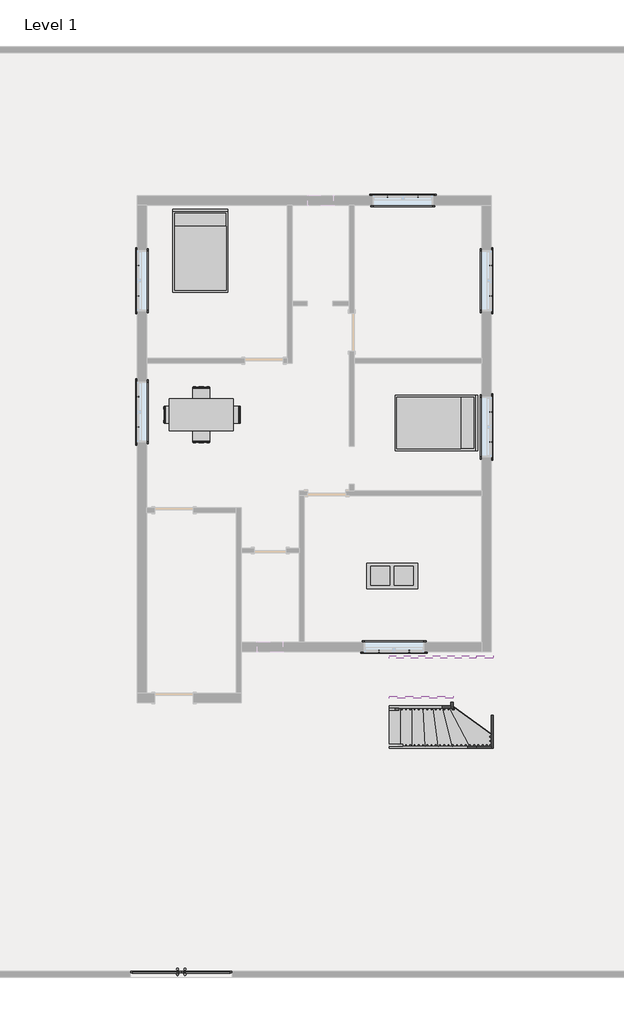
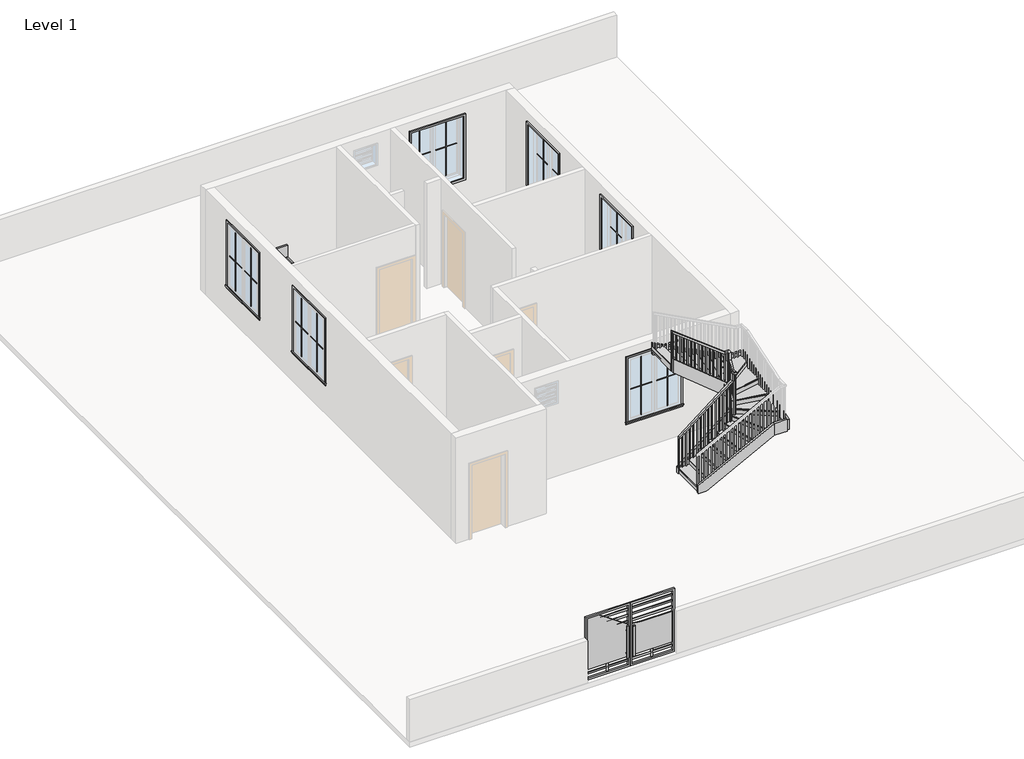
# One storey, part 3 of 3: 26 proxies, 8 members, 3 furniture elements, 1 railing, 1 stair flight.
"""IFC4 building model written with IfcOpenShell, lengths in millimetres."""

from ifc_helpers import new_model, si_unit, frame, origin, place, context, project, spatial, polyline, outline, extrude, faceted_brep, transform, mapped, element, save
from components import generic_models_113f6068, muntin_pattern_2x2_muntin_pattern_2x2_bff912c5, muntin_pattern_2x2_muntin_pattern_2x2_c2194282, trim_window_exterior_flat_with_sill_e04b3088, trim_window_interior_flat_picture_frame_2a7685fe, coffee_table_with_brass_mullions_11320_coffee_table_with_5962bef7, bed_17739_bed_17739_15c61121, dining_table_w_chairs_11374_0cdfc61b, stair_flight_c0e8b595

model = new_model("IFC4")

# Units and contexts
model_context = context("Model", 3, world=origin())
ifc_project = project(units=[si_unit("LENGTHUNIT", "METRE", prefix="MILLI")], contexts=[model_context])

# Site, building, storey
site = spatial("IfcSite", under=ifc_project)
building = spatial("IfcBuilding", under=site)
storey = spatial("IfcBuildingStorey", under=building, Name="Level 1", Elevation=0.0)

# Proxies
placement = place(None, origin())
generic_models_shape = generic_models_113f6068(model_context)
element("IfcBuildingElementProxy", 1, Name="Generic Models", at=placement, inside=storey, context=model_context, shape_type="MappedRepresentation", body=[
    mapped(generic_models_shape, transform((-4436.5644966, -12937.5476472, 0.0), x_axis=(1.0, 0.0, 0.0), y_axis=(0.0, 1.0, 0.0), z_axis=(0.0, 0.0, 1.0))),
])
muntin_pattern_2x2_muntin_pattern_2x2_shape = muntin_pattern_2x2_muntin_pattern_2x2_bff912c5(model_context)
element("IfcBuildingElementProxy", 2, Name="Muntin Pattern_2x2 : Muntin Pattern_2x2", ObjectType="Muntin Pattern_2x2 : Muntin Pattern_2x2", at=placement, inside=storey, context=model_context, shape_type="MappedRepresentation", body=[
    mapped(muntin_pattern_2x2_muntin_pattern_2x2_shape, transform((2964.3605034, 427.8534591, 984.25), x_axis=(0.0, -1.0, 0.0), y_axis=(1.0, 0.0, 0.0), z_axis=(0.0, 0.0, 1.0))),
])
element("IfcBuildingElementProxy", 3, Name="Muntin Pattern_2x2 : Muntin Pattern_2x2", ObjectType="Muntin Pattern_2x2 : Muntin Pattern_2x2", at=placement, inside=storey, context=model_context, shape_type="MappedRepresentation", body=[
    mapped(muntin_pattern_2x2_muntin_pattern_2x2_shape, transform((2964.3605034, 3923.5284591, 984.25), x_axis=(0.0, -1.0, 0.0), y_axis=(1.0, 0.0, 0.0), z_axis=(0.0, 0.0, 1.0))),
])
element("IfcBuildingElementProxy", 4, Name="Muntin Pattern_2x2 : Muntin Pattern_2x2", ObjectType="Muntin Pattern_2x2 : Muntin Pattern_2x2", at=placement, inside=storey, context=model_context, shape_type="MappedRepresentation", body=[
    mapped(muntin_pattern_2x2_muntin_pattern_2x2_shape, transform((498.9730034, 5582.4659591, 984.25), x_axis=(1.0, 0.0, 0.0), y_axis=(0.0, 1.0, 0.0), z_axis=(0.0, 0.0, 1.0))),
])
element("IfcBuildingElementProxy", 5, Name="Muntin Pattern_2x2 : Muntin Pattern_2x2", ObjectType="Muntin Pattern_2x2 : Muntin Pattern_2x2", at=placement, inside=storey, context=model_context, shape_type="MappedRepresentation", body=[
    mapped(muntin_pattern_2x2_muntin_pattern_2x2_shape, transform((-5474.7894966, 3202.8034591, 984.25), x_axis=(0.0, 1.0, 0.0), y_axis=(-1.0, 0.0, 0.0), z_axis=(0.0, 0.0, 1.0))),
])
element("IfcBuildingElementProxy", 6, Name="Muntin Pattern_2x2 : Muntin Pattern_2x2", ObjectType="Muntin Pattern_2x2 : Muntin Pattern_2x2", at=placement, inside=storey, context=model_context, shape_type="MappedRepresentation", body=[
    mapped(muntin_pattern_2x2_muntin_pattern_2x2_shape, transform((-5474.7894966, 69.0784591, 984.25), x_axis=(0.0, 1.0, 0.0), y_axis=(-1.0, 0.0, 0.0), z_axis=(0.0, 0.0, 1.0))),
])
element("IfcBuildingElementProxy", 7, Name="Muntin Pattern_2x2 : Muntin Pattern_2x2", ObjectType="Muntin Pattern_2x2 : Muntin Pattern_2x2", at=placement, inside=storey, context=model_context, shape_type="MappedRepresentation", body=[
    mapped(muntin_pattern_2x2_muntin_pattern_2x2_shape, transform((1013.3230034, -5295.0840409, 984.25), x_axis=(-1.0, 0.0, 0.0), y_axis=(0.0, -1.0, 0.0), z_axis=(0.0, 0.0, 1.0))),
])
muntin_pattern_2x2_muntin_pattern_2x2_2_shape = muntin_pattern_2x2_muntin_pattern_2x2_c2194282(model_context)
element("IfcBuildingElementProxy", 8, Name="Muntin Pattern_2x2 : Muntin Pattern_2x2", ObjectType="Muntin Pattern_2x2 : Muntin Pattern_2x2", at=placement, inside=storey, context=model_context, shape_type="MappedRepresentation", body=[
    mapped(muntin_pattern_2x2_muntin_pattern_2x2_2_shape, transform((2964.3605034, -292.8715409, 984.25), x_axis=(0.0, 1.0, 0.0), y_axis=(-1.0, 0.0, 0.0), z_axis=(0.0, 0.0, 1.0))),
])
element("IfcBuildingElementProxy", 9, Name="Muntin Pattern_2x2 : Muntin Pattern_2x2", ObjectType="Muntin Pattern_2x2 : Muntin Pattern_2x2", at=placement, inside=storey, context=model_context, shape_type="MappedRepresentation", body=[
    mapped(muntin_pattern_2x2_muntin_pattern_2x2_2_shape, transform((2964.3605034, 3202.8034591, 984.25), x_axis=(0.0, 1.0, 0.0), y_axis=(-1.0, 0.0, 0.0), z_axis=(0.0, 0.0, 1.0))),
])
element("IfcBuildingElementProxy", 10, Name="Muntin Pattern_2x2 : Muntin Pattern_2x2", ObjectType="Muntin Pattern_2x2 : Muntin Pattern_2x2", at=placement, inside=storey, context=model_context, shape_type="MappedRepresentation", body=[
    mapped(muntin_pattern_2x2_muntin_pattern_2x2_2_shape, transform((1219.6980034, 5582.4659591, 984.25), x_axis=(-1.0, 0.0, 0.0), y_axis=(0.0, -1.0, 0.0), z_axis=(0.0, 0.0, 1.0))),
])
element("IfcBuildingElementProxy", 11, Name="Muntin Pattern_2x2 : Muntin Pattern_2x2", ObjectType="Muntin Pattern_2x2 : Muntin Pattern_2x2", at=placement, inside=storey, context=model_context, shape_type="MappedRepresentation", body=[
    mapped(muntin_pattern_2x2_muntin_pattern_2x2_2_shape, transform((-5474.7894966, 3923.5284591, 984.25), x_axis=(0.0, -1.0, 0.0), y_axis=(1.0, 0.0, 0.0), z_axis=(0.0, 0.0, 1.0))),
])
element("IfcBuildingElementProxy", 12, Name="Muntin Pattern_2x2 : Muntin Pattern_2x2", ObjectType="Muntin Pattern_2x2 : Muntin Pattern_2x2", at=placement, inside=storey, context=model_context, shape_type="MappedRepresentation", body=[
    mapped(muntin_pattern_2x2_muntin_pattern_2x2_2_shape, transform((-5474.7894966, 789.8034591, 984.25), x_axis=(0.0, -1.0, 0.0), y_axis=(1.0, 0.0, 0.0), z_axis=(0.0, 0.0, 1.0))),
])
element("IfcBuildingElementProxy", 13, Name="Muntin Pattern_2x2 : Muntin Pattern_2x2", ObjectType="Muntin Pattern_2x2 : Muntin Pattern_2x2", at=placement, inside=storey, context=model_context, shape_type="MappedRepresentation", body=[
    mapped(muntin_pattern_2x2_muntin_pattern_2x2_2_shape, transform((292.5980034, -5295.0840409, 984.25), x_axis=(1.0, 0.0, 0.0), y_axis=(0.0, 1.0, 0.0), z_axis=(0.0, 0.0, 1.0))),
])
trim_window_exterior_flat_with_sill_shape = trim_window_exterior_flat_with_sill_e04b3088(model_context)
element("IfcBuildingElementProxy", 14, Name="Trim-Window-Exterior-Flat : with Sill", ObjectType="Trim-Window-Exterior-Flat : with Sill", at=placement, inside=storey, context=model_context, shape_type="MappedRepresentation", body=[
    mapped(trim_window_exterior_flat_with_sill_shape, transform((2973.8855034, 67.4909591, 2743.2), x_axis=(0.0, 1.0, 0.0), y_axis=(0.0, 0.0, 1.0), z_axis=(1.0, 0.0, 0.0))),
])
element("IfcBuildingElementProxy", 15, Name="Trim-Window-Exterior-Flat : with Sill", ObjectType="Trim-Window-Exterior-Flat : with Sill", at=placement, inside=storey, context=model_context, shape_type="MappedRepresentation", body=[
    mapped(trim_window_exterior_flat_with_sill_shape, transform((2973.8855034, 3563.1659591, 2743.2), x_axis=(0.0, 1.0, 0.0), y_axis=(0.0, 0.0, 1.0), z_axis=(1.0, 0.0, 0.0))),
])
element("IfcBuildingElementProxy", 16, Name="Trim-Window-Exterior-Flat : with Sill", ObjectType="Trim-Window-Exterior-Flat : with Sill", at=placement, inside=storey, context=model_context, shape_type="MappedRepresentation", body=[
    mapped(trim_window_exterior_flat_with_sill_shape, transform((859.3355034, 5591.9909591, 2743.2), x_axis=(-1.0, 0.0, 0.0), y_axis=(0.0, 0.0, 1.0), z_axis=(0.0, 1.0, 0.0))),
])
element("IfcBuildingElementProxy", 17, Name="Trim-Window-Exterior-Flat : with Sill", ObjectType="Trim-Window-Exterior-Flat : with Sill", at=placement, inside=storey, context=model_context, shape_type="MappedRepresentation", body=[
    mapped(trim_window_exterior_flat_with_sill_shape, transform((-5484.3144966, 3563.1659591, 2743.2), x_axis=(0.0, -1.0, 0.0), y_axis=(0.0, 0.0, 1.0), z_axis=(-1.0, 0.0, 0.0))),
])
element("IfcBuildingElementProxy", 18, Name="Trim-Window-Exterior-Flat : with Sill", ObjectType="Trim-Window-Exterior-Flat : with Sill", at=placement, inside=storey, context=model_context, shape_type="MappedRepresentation", body=[
    mapped(trim_window_exterior_flat_with_sill_shape, transform((-5484.3144966, 429.4409591, 2743.2), x_axis=(0.0, -1.0, 0.0), y_axis=(0.0, 0.0, 1.0), z_axis=(-1.0, 0.0, 0.0))),
])
element("IfcBuildingElementProxy", 19, Name="Trim-Window-Exterior-Flat : with Sill", ObjectType="Trim-Window-Exterior-Flat : with Sill", at=placement, inside=storey, context=model_context, shape_type="MappedRepresentation", body=[
    mapped(trim_window_exterior_flat_with_sill_shape, transform((652.9605034, -5304.6090409, 2743.2), x_axis=(1.0, 0.0, 0.0), y_axis=(0.0, 0.0, 1.0), z_axis=(0.0, -1.0, 0.0))),
])
trim_window_interior_flat_picture_frame_shape = trim_window_interior_flat_picture_frame_2a7685fe(model_context)
element("IfcBuildingElementProxy", 20, Name="Trim-Window-Interior-Flat : Picture Frame", ObjectType="Trim-Window-Interior-Flat : Picture Frame", at=placement, inside=storey, context=model_context, shape_type="MappedRepresentation", body=[
    mapped(trim_window_interior_flat_picture_frame_shape, transform((2745.2855034, 67.4909591, 2743.2), x_axis=(0.0, -1.0, 0.0), y_axis=(0.0, 0.0, 1.0), z_axis=(-1.0, 0.0, 0.0))),
])
element("IfcBuildingElementProxy", 21, Name="Trim-Window-Interior-Flat : Picture Frame", ObjectType="Trim-Window-Interior-Flat : Picture Frame", at=placement, inside=storey, context=model_context, shape_type="MappedRepresentation", body=[
    mapped(trim_window_interior_flat_picture_frame_shape, transform((2745.2855034, 3563.1659591, 2743.2), x_axis=(0.0, -1.0, 0.0), y_axis=(0.0, 0.0, 1.0), z_axis=(-1.0, 0.0, 0.0))),
])
element("IfcBuildingElementProxy", 22, Name="Trim-Window-Interior-Flat : Picture Frame", ObjectType="Trim-Window-Interior-Flat : Picture Frame", at=placement, inside=storey, context=model_context, shape_type="MappedRepresentation", body=[
    mapped(trim_window_interior_flat_picture_frame_shape, transform((859.3355034, 5363.3909591, 2743.2), x_axis=(1.0, 0.0, 0.0), y_axis=(0.0, 0.0, 1.0), z_axis=(0.0, -1.0, 0.0))),
])
element("IfcBuildingElementProxy", 23, Name="Trim-Window-Interior-Flat : Picture Frame", ObjectType="Trim-Window-Interior-Flat : Picture Frame", at=placement, inside=storey, context=model_context, shape_type="MappedRepresentation", body=[
    mapped(trim_window_interior_flat_picture_frame_shape, transform((-5255.7144966, 3563.1659591, 2743.2), x_axis=(0.0, 1.0, 0.0), y_axis=(0.0, 0.0, 1.0), z_axis=(1.0, 0.0, 0.0))),
])
element("IfcBuildingElementProxy", 24, Name="Trim-Window-Interior-Flat : Picture Frame", ObjectType="Trim-Window-Interior-Flat : Picture Frame", at=placement, inside=storey, context=model_context, shape_type="MappedRepresentation", body=[
    mapped(trim_window_interior_flat_picture_frame_shape, transform((-5255.7144966, 429.4409591, 2743.2), x_axis=(0.0, 1.0, 0.0), y_axis=(0.0, 0.0, 1.0), z_axis=(1.0, 0.0, 0.0))),
])
element("IfcBuildingElementProxy", 25, Name="Trim-Window-Interior-Flat : Picture Frame", ObjectType="Trim-Window-Interior-Flat : Picture Frame", at=placement, inside=storey, context=model_context, shape_type="MappedRepresentation", body=[
    mapped(trim_window_interior_flat_picture_frame_shape, transform((652.9605034, -5076.0090409, 2743.2), x_axis=(-1.0, 0.0, 0.0), y_axis=(0.0, 0.0, 1.0), z_axis=(0.0, 1.0, 0.0))),
])
coffee_table_with_brass_mullions_11320_coffee_table_with_shape = coffee_table_with_brass_mullions_11320_coffee_table_with_5962bef7(model_context)
element("IfcBuildingElementProxy", 26, Name="coffee_table_with_brass_mullions_11320 : coffee_table_with_brass_mullions_11320", ObjectType="coffee_table_with_brass_mullions_11320 : coffee_table_with_brass_mullions_11320", at=placement, inside=storey, context=model_context, shape_type="MappedRepresentation", body=[
    mapped(coffee_table_with_brass_mullions_11320_coffee_table_with_shape, transform((1240.0943553, -3926.0808329, 0.0), x_axis=(1.0, 0.0, 0.0), y_axis=(0.0, 1.0, 0.0), z_axis=(0.0, 0.0, 1.0))),
])

# Furniture
bed_17739_bed_17739_shape = bed_17739_bed_17739_15c61121(model_context)
element("IfcFurniture", 27, ObjectType="Bed_17739 : Bed_17739", at=placement, inside=storey, context=model_context, shape_type="MappedRepresentation", body=[
    mapped(bed_17739_bed_17739_shape, transform((-3979.3644966, 4258.4909591, 0.0), x_axis=(1.0, 0.0, 0.0), y_axis=(0.0, 1.0, 0.0), z_axis=(0.0, 0.0, 1.0))),
])
element("IfcFurniture", 28, ObjectType="Bed_17739 : Bed_17739", at=placement, inside=storey, context=model_context, shape_type="MappedRepresentation", body=[
    mapped(bed_17739_bed_17739_shape, transform((1640.3855034, 162.7409591, 0.0), x_axis=(0.0, -1.0, 0.0), y_axis=(1.0, 0.0, 0.0), z_axis=(0.0, 0.0, 1.0))),
])
dining_table_w_chairs_11374_shape = dining_table_w_chairs_11374_0cdfc61b(model_context)
element("IfcFurniture", 29, ObjectType="Dining_Table_w_Chairs_11374", at=placement, inside=storey, context=model_context, shape_type="MappedRepresentation", body=[
    mapped(dining_table_w_chairs_11374_shape, transform((-3975.2132663, 265.1952874, 0.0), x_axis=(1.0, 0.0, 0.0), y_axis=(0.0, 1.0, 0.0), z_axis=(0.0, 0.0, 1.0))),
])

# Members
element("IfcMember", 30, ObjectType="Stringer - 2\" Width", at=placement, inside=storey, context=model_context, shape_type="SweptSolid", body=[
    extrude(outline(polyline([(176.1764461, 531.7538115), (0.0, 531.7538115), (0.0, 798.0154561), (987.1410923, 2008.6855034), (1380.418648, 2008.6855034), (176.1764461, 531.7538115)])), frame((0.0, -6650.8090409, 0.0), z_axis=(0.0, 1.0, 0.0), x_axis=(0.0, 0.0, 1.0)), (0.0, 0.0, 1.0), 50.8),
])
element("IfcMember", 31, ObjectType="Stringer - 2\" Width", at=placement, inside=storey, context=model_context, shape_type="SweptSolid", body=[
    extrude(outline(polyline([(-6650.8090409, 1028.5617647), (-6650.8090409, 1573.2682978), (-6444.1719234, 1926.1409689), (-6422.2090409, 1926.1409689), (-6422.2090409, 1360.465107), (-6616.5668235, 1028.5617647), (-6650.8090409, 1028.5617647)])), frame((2008.6855034, 0.0, 0.0), z_axis=(1.0, 0.0, 0.0), x_axis=(0.0, 1.0, 0.0)), (0.0, 0.0, 1.0), 50.8),
])
element("IfcMember", 32, ObjectType="Stringer - 2\" Width", at=placement, inside=storey, context=model_context, shape_type="SweptSolid", body=[
    extrude(outline(polyline([(1532.8634131, 2059.4855034), (1926.1409689, 2059.4855034), (3171.8038432, 531.7538115), (2778.5262875, 531.7538115), (1532.8634131, 2059.4855034)])), frame((0.0, -6422.2090409, 0.0), z_axis=(0.0, 1.0, 0.0), x_axis=(0.0, 0.0, 1.0)), (0.0, 0.0, 1.0), 50.8),
])
element("IfcMember", 33, ObjectType="Stringer - 2\" Width", at=placement, inside=storey, context=model_context, shape_type="SweptSolid", body=[
    extrude(outline(polyline([(229.639954, 531.7538115), (0.0, 531.7538115), (0.0, 751.5161291), (962.500629, 2619.1710032), (1305.3956453, 2619.1710032), (229.639954, 531.7538115)])), frame((0.0, -7616.0090409, 0.0), z_axis=(0.0, 1.0, 0.0), x_axis=(0.0, 0.0, 1.0)), (0.0, 0.0, 1.0), 50.8),
])
element("IfcMember", 34, ObjectType="Stringer - 2\" Width", at=placement, inside=storey, context=model_context, shape_type="SweptSolid", body=[
    extrude(outline(polyline([(2619.1710032, -7616.0090409), (2619.1710032, -7565.2090409), (2973.8855034, -7565.2090409), (2973.8855034, -7616.0090409), (2619.1710032, -7616.0090409)])), frame((0.0, 0.0, 962.500629), z_axis=(0.0, 0.0, 1.0), x_axis=(1.0, 0.0, 0.0)), (0.0, 0.0, 1.0), 342.8950162),
])
element("IfcMember", 35, ObjectType="Stringer - 2\" Width", at=placement, inside=storey, context=model_context, shape_type="SweptSolid", body=[
    extrude(outline(polyline([(-7616.0090409, 1000.5956453), (-7616.0090409, 1289.0952212), (-5493.9891581, 1969.9972697), (-5457.0090409, 1969.9972697), (-5457.0090409, 1638.9682298), (-7446.4865579, 1000.5956453), (-7616.0090409, 1000.5956453)])), frame((2973.8855034, 0.0, 0.0), z_axis=(1.0, 0.0, 0.0), x_axis=(0.0, 1.0, 0.0)), (0.0, 0.0, 1.0), 50.8),
])
element("IfcMember", 36, ObjectType="Stringer - 2\" Width", at=placement, inside=storey, context=model_context, shape_type="SweptSolid", body=[
    extrude(outline(polyline([(3024.6855034, -5406.2090409), (3024.6855034, -5457.0090409), (2619.1710032, -5457.0090409), (2619.1710032, -5406.2090409), (3024.6855034, -5406.2090409)])), frame((0.0, 0.0, 1649.8904473), z_axis=(0.0, 0.0, 1.0), x_axis=(1.0, 0.0, 0.0)), (0.0, 0.0, 1.0), 320.1068224),
])
element("IfcMember", 37, ObjectType="Stringer - 2\" Width", at=placement, inside=storey, context=model_context, shape_type="SweptSolid", body=[
    extrude(outline(polyline([(1649.8904473, 2619.1710032), (1969.9972697, 2619.1710032), (3045.7529609, 531.7538115), (2725.6461385, 531.7538115), (1649.8904473, 2619.1710032)])), frame((0.0, -5457.0090409, 0.0), z_axis=(0.0, 1.0, 0.0), x_axis=(0.0, 0.0, 1.0)), (0.0, 0.0, 1.0), 50.8),
])

# Railing
element("IfcRailing", 38, ObjectType="Handrail - Rectangular", at=placement, inside=storey, context=model_context, shape_type="SolidModel", body=[
    faceted_brep([(531.7538115, -6650.8090409, 1083.7333333), (531.7538115, -6650.8090409, 1019.4000346), (531.7538115, -6701.6090409, 1019.4000346), (531.7538115, -6701.6090409, 1083.7333333), (1983.2855034, -6650.8090409, 2211.6191036), (2034.0855034, -6650.8090409, 2186.7590024), (2034.0855034, -6701.6090409, 2186.7590024), (1983.2855034, -6701.6090409, 2211.6191036), (2059.4855034, -6545.487707, 2363.8281882), (2059.4855034, -6574.6090409, 2414.6281882), (2059.4855034, -6447.6090409, 2631.5051451), (2059.4855034, -6396.8090409, 2617.7256424), (2110.2855034, -6545.487707, 2363.8281882), (2110.2855034, -6396.8090409, 2617.7256424), (2110.2855034, -6574.6090409, 2414.6281882), (2110.2855034, -6447.6090409, 2631.5051451), (531.7538115, -6371.4090409, 3962.4), (531.7538115, -6320.6090409, 3962.4), (531.7538115, -6320.6090409, 3898.0667013), (531.7538115, -6371.4090409, 3898.0667013), (1965.8688354, -6371.4090409, 2783.7142297), (1983.2855034, -6371.4090409, 2834.5142297), (1965.8688354, -6320.6090409, 2783.7142297), (1983.2855034, -6320.6090409, 2834.5142297), (1983.2855034, -6650.8090409, 2414.6281882), (2034.0855034, -6650.8090409, 2363.8281882), (2034.0855034, -6701.6090409, 2363.8281882), (1983.2855034, -6701.6090409, 2414.6281882), (2059.4855034, -6650.8090409, 2414.6281882), (2059.4855034, -6650.8090409, 2363.8281882), (2110.2855034, -6701.6090409, 2363.8281882), (2110.2855034, -6701.6090409, 2414.6281882), (2059.4855034, -6447.6090409, 2834.5142297), (2059.4855034, -6396.8090409, 2783.7142297), (2110.2855034, -6396.8090409, 2783.7142297), (2110.2855034, -6447.6090409, 2834.5142297), (2059.4855034, -6371.4090409, 2834.5142297), (2059.4855034, -6371.4090409, 2783.7142297), (2110.2855034, -6320.6090409, 2783.7142297), (2110.2855034, -6320.6090409, 2834.5142297)], [[[0, 1, 2, 3]], [[1, 0, 4, 5]], [[2, 1, 5, 6]], [[3, 2, 6, 7]], [[0, 3, 7, 4]], [[8, 9, 10, 11]], [[12, 8, 11, 13]], [[14, 12, 13, 15]], [[9, 14, 15, 10]], [[16, 17, 18, 19]], [[20, 21, 16, 19]], [[22, 20, 19, 18]], [[23, 22, 18, 17]], [[21, 23, 17, 16]], [[5, 4, 24, 25]], [[6, 5, 25, 26]], [[7, 6, 26, 27]], [[4, 7, 27, 24]], [[25, 24, 28, 29]], [[26, 25, 29, 30]], [[27, 26, 30, 31]], [[24, 27, 31, 28]], [[29, 28, 9, 8]], [[30, 29, 8, 12]], [[31, 30, 12, 14]], [[28, 31, 14, 9]], [[11, 10, 32, 33]], [[13, 11, 33, 34]], [[15, 13, 34, 35]], [[10, 15, 35, 32]], [[33, 32, 36, 37]], [[34, 33, 37, 38]], [[35, 34, 38, 39]], [[32, 35, 39, 36]], [[37, 36, 21, 20]], [[38, 37, 20, 22]], [[39, 38, 22, 23]], [[36, 39, 23, 21]]]),
    extrude(outline(polyline([(3882.8316852, 551.3605034), (2878.6666667, 551.3605034), (2878.6666667, 570.4105034), (3868.0292361, 570.4105034), (3882.8316852, 551.3605034)])), frame((0.0, -6355.5340409, 0.0), z_axis=(0.0, 1.0, 0.0), x_axis=(0.0, 0.0, 1.0)), (0.0, 0.0, 1.0), 19.05),
    extrude(outline(polyline([(3803.8852902, 652.9605034), (2878.6666667, 652.9605034), (2878.6666667, 672.0105034), (3789.0828411, 672.0105034), (3803.8852902, 652.9605034)])), frame((0.0, -6355.5340409, 0.0), z_axis=(0.0, 1.0, 0.0), x_axis=(0.0, 0.0, 1.0)), (0.0, 0.0, 1.0), 19.05),
    extrude(outline(polyline([(3724.9388952, 754.5605034), (2878.6666667, 754.5605034), (2878.6666667, 773.6105034), (3710.1364462, 773.6105034), (3724.9388952, 754.5605034)])), frame((0.0, -6355.5340409, 0.0), z_axis=(0.0, 1.0, 0.0), x_axis=(0.0, 0.0, 1.0)), (0.0, 0.0, 1.0), 19.05),
    extrude(outline(polyline([(3645.9925003, 856.1605034), (2709.3333333, 856.1605034), (2709.3333333, 875.2105034), (3631.1900512, 875.2105034), (3645.9925003, 856.1605034)])), frame((0.0, -6355.5340409, 0.0), z_axis=(0.0, 1.0, 0.0), x_axis=(0.0, 0.0, 1.0)), (0.0, 0.0, 1.0), 19.05),
    extrude(outline(polyline([(3567.0461053, 957.7605034), (2709.3333333, 957.7605034), (2709.3333333, 976.8105034), (3552.2436562, 976.8105034), (3567.0461053, 957.7605034)])), frame((0.0, -6355.5340409, 0.0), z_axis=(0.0, 1.0, 0.0), x_axis=(0.0, 0.0, 1.0)), (0.0, 0.0, 1.0), 19.05),
    extrude(outline(polyline([(3488.0997103, 1059.3605034), (2709.3333333, 1059.3605034), (2709.3333333, 1078.4105034), (3473.2972613, 1078.4105034), (3488.0997103, 1059.3605034)])), frame((0.0, -6355.5340409, 0.0), z_axis=(0.0, 1.0, 0.0), x_axis=(0.0, 0.0, 1.0)), (0.0, 0.0, 1.0), 19.05),
    extrude(outline(polyline([(3409.1533154, 1160.9605034), (2540.0, 1160.9605034), (2540.0, 1180.0105034), (3394.3508663, 1180.0105034), (3409.1533154, 1160.9605034)])), frame((0.0, -6355.5340409, 0.0), z_axis=(0.0, 1.0, 0.0), x_axis=(0.0, 0.0, 1.0)), (0.0, 0.0, 1.0), 19.05),
    extrude(outline(polyline([(3330.2069204, 1262.5605034), (2540.0, 1262.5605034), (2540.0, 1281.6105034), (3315.4044713, 1281.6105034), (3330.2069204, 1262.5605034)])), frame((0.0, -6355.5340409, 0.0), z_axis=(0.0, 1.0, 0.0), x_axis=(0.0, 0.0, 1.0)), (0.0, 0.0, 1.0), 19.05),
    extrude(outline(polyline([(3251.2605254, 1364.1605034), (2370.6666667, 1364.1605034), (2370.6666667, 1383.2105034), (3236.4580764, 1383.2105034), (3251.2605254, 1364.1605034)])), frame((0.0, -6355.5340409, 0.0), z_axis=(0.0, 1.0, 0.0), x_axis=(0.0, 0.0, 1.0)), (0.0, 0.0, 1.0), 19.05),
    extrude(outline(polyline([(3172.3141304, 1465.7605034), (2370.6666667, 1465.7605034), (2370.6666667, 1484.8105034), (3157.5116814, 1484.8105034), (3172.3141304, 1465.7605034)])), frame((0.0, -6355.5340409, 0.0), z_axis=(0.0, 1.0, 0.0), x_axis=(0.0, 0.0, 1.0)), (0.0, 0.0, 1.0), 19.05),
    extrude(outline(polyline([(3093.3677355, 1567.3605034), (2370.6666667, 1567.3605034), (2370.6666667, 1586.4105034), (3078.5652864, 1586.4105034), (3093.3677355, 1567.3605034)])), frame((0.0, -6355.5340409, 0.0), z_axis=(0.0, 1.0, 0.0), x_axis=(0.0, 0.0, 1.0)), (0.0, 0.0, 1.0), 19.05),
    extrude(outline(polyline([(3014.4213405, 1668.9605034), (2201.3333333, 1668.9605034), (2201.3333333, 1688.0105034), (2999.6188914, 1688.0105034), (3014.4213405, 1668.9605034)])), frame((0.0, -6355.5340409, 0.0), z_axis=(0.0, 1.0, 0.0), x_axis=(0.0, 0.0, 1.0)), (0.0, 0.0, 1.0), 19.05),
    extrude(outline(polyline([(2935.4749455, 1770.5605034), (2201.3333333, 1770.5605034), (2201.3333333, 1789.6105034), (2920.6724965, 1789.6105034), (2935.4749455, 1770.5605034)])), frame((0.0, -6355.5340409, 0.0), z_axis=(0.0, 1.0, 0.0), x_axis=(0.0, 0.0, 1.0)), (0.0, 0.0, 1.0), 19.05),
    extrude(outline(polyline([(2856.5285506, 1872.1605034), (2032.0, 1872.1605034), (2032.0, 1891.2105034), (2841.7261015, 1891.2105034), (2856.5285506, 1872.1605034)])), frame((0.0, -6355.5340409, 0.0), z_axis=(0.0, 1.0, 0.0), x_axis=(0.0, 0.0, 1.0)), (0.0, 0.0, 1.0), 19.05),
    extrude(outline(polyline([(2777.5821556, 1973.7605034), (2032.0, 1973.7605034), (2032.0, 1992.8105034), (2762.7797065, 1992.8105034), (2777.5821556, 1973.7605034)])), frame((0.0, -6355.5340409, 0.0), z_axis=(0.0, 1.0, 0.0), x_axis=(0.0, 0.0, 1.0)), (0.0, 0.0, 1.0), 19.05),
    extrude(outline(polyline([(2075.3605034, -6380.9340409), (2075.3605034, -6361.8840409), (2094.4105034, -6361.8840409), (2094.4105034, -6380.9340409), (2075.3605034, -6380.9340409)])), frame((0.0, 0.0, 1693.3333333), z_axis=(0.0, 0.0, 1.0), x_axis=(1.0, 0.0, 0.0)), (0.0, 0.0, 1.0), 1090.3808964),
    extrude(outline(polyline([(-6463.4840409, 2503.86524), (-6463.4840409, 1524.0), (-6482.5340409, 1524.0), (-6482.5340409, 2471.3336964), (-6463.4840409, 2503.86524)])), frame((2075.3605034, 0.0, 0.0), z_axis=(1.0, 0.0, 0.0), x_axis=(0.0, 1.0, 0.0)), (0.0, 0.0, 1.0), 19.05),
    extrude(outline(polyline([(-6565.0840409, 2330.3636744), (-6565.0840409, 1354.6666667), (-6584.1340409, 1354.6666667), (-6584.1340409, 2297.8321309), (-6565.0840409, 2330.3636744)])), frame((2075.3605034, 0.0, 0.0), z_axis=(1.0, 0.0, 0.0), x_axis=(0.0, 1.0, 0.0)), (0.0, 0.0, 1.0), 19.05),
    extrude(outline(polyline([(2046.2288115, -6666.6840409), (2065.2788115, -6666.6840409), (2065.2788115, -6685.7340409), (2046.2288115, -6685.7340409), (2046.2288115, -6666.6840409)])), frame((0.0, 0.0, 1185.3333333), z_axis=(0.0, 0.0, 1.0), x_axis=(1.0, 0.0, 0.0)), (0.0, 0.0, 1.0), 1178.4948549),
    extrude(outline(polyline([(2117.2483397, 1944.6288115), (1016.0, 1944.6288115), (1016.0, 1963.6788115), (2132.0507888, 1963.6788115), (2117.2483397, 1944.6288115)])), frame((0.0, -6685.7340409, 0.0), z_axis=(0.0, 1.0, 0.0), x_axis=(0.0, 0.0, 1.0)), (0.0, 0.0, 1.0), 19.05),
    extrude(outline(polyline([(2038.3019447, 1843.0288115), (1016.0, 1843.0288115), (1016.0, 1862.0788115), (2053.1043938, 1862.0788115), (2038.3019447, 1843.0288115)])), frame((0.0, -6685.7340409, 0.0), z_axis=(0.0, 1.0, 0.0), x_axis=(0.0, 0.0, 1.0)), (0.0, 0.0, 1.0), 19.05),
    extrude(outline(polyline([(1959.3555498, 1741.4288115), (846.6666667, 1741.4288115), (846.6666667, 1760.4788115), (1974.1579988, 1760.4788115), (1959.3555498, 1741.4288115)])), frame((0.0, -6685.7340409, 0.0), z_axis=(0.0, 1.0, 0.0), x_axis=(0.0, 0.0, 1.0)), (0.0, 0.0, 1.0), 19.05),
    extrude(outline(polyline([(1880.4091548, 1639.8288115), (846.6666667, 1639.8288115), (846.6666667, 1658.8788115), (1895.2116039, 1658.8788115), (1880.4091548, 1639.8288115)])), frame((0.0, -6685.7340409, 0.0), z_axis=(0.0, 1.0, 0.0), x_axis=(0.0, 0.0, 1.0)), (0.0, 0.0, 1.0), 19.05),
    extrude(outline(polyline([(1801.4627598, 1538.2288115), (677.3333333, 1538.2288115), (677.3333333, 1557.2788115), (1816.2652089, 1557.2788115), (1801.4627598, 1538.2288115)])), frame((0.0, -6685.7340409, 0.0), z_axis=(0.0, 1.0, 0.0), x_axis=(0.0, 0.0, 1.0)), (0.0, 0.0, 1.0), 19.05),
    extrude(outline(polyline([(1722.5163649, 1436.6288115), (677.3333333, 1436.6288115), (677.3333333, 1455.6788115), (1737.3188139, 1455.6788115), (1722.5163649, 1436.6288115)])), frame((0.0, -6685.7340409, 0.0), z_axis=(0.0, 1.0, 0.0), x_axis=(0.0, 0.0, 1.0)), (0.0, 0.0, 1.0), 19.05),
    extrude(outline(polyline([(1643.5699699, 1335.0288115), (508.0, 1335.0288115), (508.0, 1354.0788115), (1658.3724189, 1354.0788115), (1643.5699699, 1335.0288115)])), frame((0.0, -6685.7340409, 0.0), z_axis=(0.0, 1.0, 0.0), x_axis=(0.0, 0.0, 1.0)), (0.0, 0.0, 1.0), 19.05),
    extrude(outline(polyline([(1564.6235749, 1233.4288115), (508.0, 1233.4288115), (508.0, 1252.4788115), (1579.426024, 1252.4788115), (1564.6235749, 1233.4288115)])), frame((0.0, -6685.7340409, 0.0), z_axis=(0.0, 1.0, 0.0), x_axis=(0.0, 0.0, 1.0)), (0.0, 0.0, 1.0), 19.05),
    extrude(outline(polyline([(1485.6771799, 1131.8288115), (508.0, 1131.8288115), (508.0, 1150.8788115), (1500.479629, 1150.8788115), (1485.6771799, 1131.8288115)])), frame((0.0, -6685.7340409, 0.0), z_axis=(0.0, 1.0, 0.0), x_axis=(0.0, 0.0, 1.0)), (0.0, 0.0, 1.0), 19.05),
    extrude(outline(polyline([(1406.730785, 1030.2288115), (338.6666667, 1030.2288115), (338.6666667, 1049.2788115), (1421.533234, 1049.2788115), (1406.730785, 1030.2288115)])), frame((0.0, -6685.7340409, 0.0), z_axis=(0.0, 1.0, 0.0), x_axis=(0.0, 0.0, 1.0)), (0.0, 0.0, 1.0), 19.05),
    extrude(outline(polyline([(1327.78439, 928.6288115), (338.6666667, 928.6288115), (338.6666667, 947.6788115), (1342.5868391, 947.6788115), (1327.78439, 928.6288115)])), frame((0.0, -6685.7340409, 0.0), z_axis=(0.0, 1.0, 0.0), x_axis=(0.0, 0.0, 1.0)), (0.0, 0.0, 1.0), 19.05),
    extrude(outline(polyline([(1248.837995, 827.0288115), (338.6666667, 827.0288115), (338.6666667, 846.0788115), (1263.6404441, 846.0788115), (1248.837995, 827.0288115)])), frame((0.0, -6685.7340409, 0.0), z_axis=(0.0, 1.0, 0.0), x_axis=(0.0, 0.0, 1.0)), (0.0, 0.0, 1.0), 19.05),
    extrude(outline(polyline([(1169.8916001, 725.4288115), (169.3333333, 725.4288115), (169.3333333, 744.4788115), (1184.6940491, 744.4788115), (1169.8916001, 725.4288115)])), frame((0.0, -6685.7340409, 0.0), z_axis=(0.0, 1.0, 0.0), x_axis=(0.0, 0.0, 1.0)), (0.0, 0.0, 1.0), 19.05),
    extrude(outline(polyline([(1090.9452051, 623.8288115), (169.3333333, 623.8288115), (169.3333333, 642.8788115), (1105.7476541, 642.8788115), (1090.9452051, 623.8288115)])), frame((0.0, -6685.7340409, 0.0), z_axis=(0.0, 1.0, 0.0), x_axis=(0.0, 0.0, 1.0)), (0.0, 0.0, 1.0), 19.05),
    extrude(outline(polyline([(2075.3605034, -6355.5340409), (2075.3605034, -6336.4840409), (2094.4105034, -6336.4840409), (2094.4105034, -6355.5340409), (2075.3605034, -6355.5340409)])), frame((0.0, 0.0, 1862.6666667), z_axis=(0.0, 0.0, 1.0), x_axis=(1.0, 0.0, 0.0)), (0.0, 0.0, 1.0), 921.0475631),
    extrude(outline(polyline([(2075.3605034, -6666.6840409), (2094.4105034, -6666.6840409), (2094.4105034, -6685.7340409), (2075.3605034, -6685.7340409), (2075.3605034, -6666.6840409)])), frame((0.0, 0.0, 1185.3333333), z_axis=(0.0, 0.0, 1.0), x_axis=(1.0, 0.0, 0.0)), (0.0, 0.0, 1.0), 1178.4948549),
    extrude(outline(polyline([(3898.0667013, 531.7538115), (2878.6666667, 531.7538115), (2878.6666667, 550.8038115), (3883.2642523, 550.8038115), (3898.0667013, 531.7538115)])), frame((0.0, -6355.5340409, 0.0), z_axis=(0.0, 1.0, 0.0), x_axis=(0.0, 0.0, 1.0)), (0.0, 0.0, 1.0), 19.05),
    extrude(outline(polyline([(1019.4000346, 531.7538115), (169.3333333, 531.7538115), (169.3333333, 550.8038115), (1034.2024837, 550.8038115), (1019.4000346, 531.7538115)])), frame((0.0, -6685.7340409, 0.0), z_axis=(0.0, 1.0, 0.0), x_axis=(0.0, 0.0, 1.0)), (0.0, 0.0, 1.0), 19.05),
])

# Stair flight
stair_flight_shape = stair_flight_c0e8b595(model_context)
element("IfcStairFlight", 39, ObjectType="2\" Tread 1\" Nosing 1/4\" Riser", at=placement, inside=storey, context=model_context, shape_type="MappedRepresentation", body=[
    mapped(stair_flight_shape, transform((0.0, 0.0, 0.0), x_axis=(1.0, 0.0, 0.0), y_axis=(0.0, 1.0, 0.0), z_axis=(0.0, 0.0, 1.0))),
])

save(model, "model.ifc")

# Revit data of these elements
# Type
#   sheet = none
#   pipe = none
#   handal = none
#   faram = none
#   Default Elevation = 0
# Type "Muntin Pattern_2x2 : Muntin Pattern_2x2"
#   Width [instance default] = 4' - 0"
#   Thickness = 0' - 0 1/2"
#   Height [instance default] = 4' - 0"
#   Distance = 0' - 0 3/4"
#   Interior Material [instance default] = none
#   Exterior Material [instance default] = none
#   Default Elevation = 0
# Type "Trim-Window-Exterior-Flat : with Sill"
#   Trim Width = 0' - 2 1/4"
#   Trim Thickness_Picture Frame = 0' - 1 1/4"
#   Trim Thickness_with Sill = 0' - 0 3/4"
#   Sill Thickness = 0' - 1 1/4"
#   Opening Width [instance default] = 2' - 0"
#   Opening Height [instance default] = 3' - 0"
#   Default Elevation = 4' - 0"
#   Sill = yes
#   Picture Frame = no
#   Trim Material [instance default] = none
# Type "Trim-Window-Interior-Flat : Picture Frame"
#   Trim Thickness_Picture Frame = 0' - 1 1/4"
#   Trim Width = 0' - 2 1/4"
#   Trim Thickness_with Sill = 0' - 0 3/4"
#   Sill Thickness = 0' - 1 1/4"
#   Opening Width [instance default] = 2' - 0"
#   Opening Height [instance default] = 3' - 0"
#   Default Elevation = 4' - 0"
#   Sill = no
#   Picture Frame = yes
#   Trim Material [instance default] = none
# Type "coffee_table_with_brass_mullions_11320 : coffee_table_with_brass_mullions_11320"
#   Default Elevation = 0
# Type "Bed_17739 : Bed_17739"
#   Default Elevation = 0
# Type "Dining_Table_w_Chairs_11374"
#   Default Elevation = 0
#   Assembly Code = ""
# Type "Handrail - Rectangular"
#   Assembly Code = "C2010400"
#   built-in parameter 1008612 = 0.0416667 (stored number, unit not read)
#   built-in parameter 1008611 = 0.0416667 (stored number, unit not read)
#   built-in parameter 1008609 = 0.333333 (stored number, unit not read)
#   built-in parameter 1008604 = 0.166667 (stored number, unit not read)
#   built-in parameter 1008603 = 0.166667 (stored number, unit not read)
#   Railing Height = 3' - 0"
#   built-in parameter 1008630 = 2
#   built-in parameter 1008610 = 2
#   built-in parameter 1008618 = Baluster - Square : 3/4"
# Element 1 (IfcBuildingElementProxy)
#   Phase Created = New Construction
# Elements 2, 3, 4, 5, 6, 7, 8, 9, 10, 11, 12, 13 (IfcBuildingElementProxy, "Muntin Pattern_2x2 : Muntin Pattern_2x2")
#   Width = 1' - 11 1/8"
#   Height = 5' - 6 1/2"
#   Interior Material = Wood - Stained
#   Exterior Material = Clad - White
#   Phase Created = New Construction
#   Materials on its faces: "Clad - White", "Wood - Stained"
# Elements 14, 15, 16, 17, 18, 19 (IfcBuildingElementProxy, "Trim-Window-Exterior-Flat : with Sill")
#   Opening Width = 4' - 9"
#   Opening Height = 6' - 0"
#   Trim Material = Clad - White
#   Phase Created = New Construction
#   Materials on its faces: "Clad - White"
# Elements 20, 21, 22, 23, 24, 25 (IfcBuildingElementProxy, "Trim-Window-Interior-Flat : Picture Frame")
#   Opening Width = 4' - 9"
#   Opening Height = 6' - 0"
#   Trim Material = Wood - Stained
#   Phase Created = New Construction
#   Materials on its faces: "Wood - Stained"
# Element 26 (IfcBuildingElementProxy, "coffee_table_with_brass_mullions_11320 : coffee_table_with_brass_mullions_11320")
#   Phase Created = New Construction
#   Materials on its faces: "Default Wall", "TABLE", "Glass", "Default"
# Elements 27, 28 (IfcFurniture, "Bed_17739 : Bed_17739")
#   Phase Created = New Construction
#   Materials on its faces: "legs", "sheets", "bed frame", "Blanket"
# Element 29 (IfcFurniture, "Dining_Table_w_Chairs_11374")
#   Phase Created = New Construction
# Elements 30, 31, 32, 33, 34, 35, 36, 37 (IfcMember, "Stringer - 2\" Width")
#   Phase Created = New Construction
# Element 38 (IfcRailing, "Handrail - Rectangular")
#   Phase Created = New Construction
# Element 39 (IfcStairFlight, "2\" Tread 1\" Nosing 1/4\" Riser")
#   Phase Created = New Construction
# Materials
#   "Clad - White": class "Wood", colour RGB 242 242 238, transparency 0, Cost = 0
#   "Wood - Stained": class "Wood", colour RGB 224 178 126, transparency 0, Cost = 0
#   "Default Wall": colour RGB 128 128 128, transparency 0, Cost = 0
#   "TABLE": class "Generic", colour RGB 120 120 120, transparency 0, Cost = 0
#   "Glass": class "Glass", colour RGB 0 128 192, transparency 0.75, Description = "Soda Lime Glass", Cost = 0
#   "Default": colour RGB 127 127 127, transparency 0, Cost = 0
#   "legs": colour RGB 90 73 37, transparency 0, Cost = 0
#   "sheets": colour RGB 200 195 176, transparency 0, Cost = 0
#   "bed frame": colour RGB 90 73 37, transparency 0, Cost = 0
#   "Blanket": class "System", colour RGB 59 0 1, transparency 0, Cost = 0
